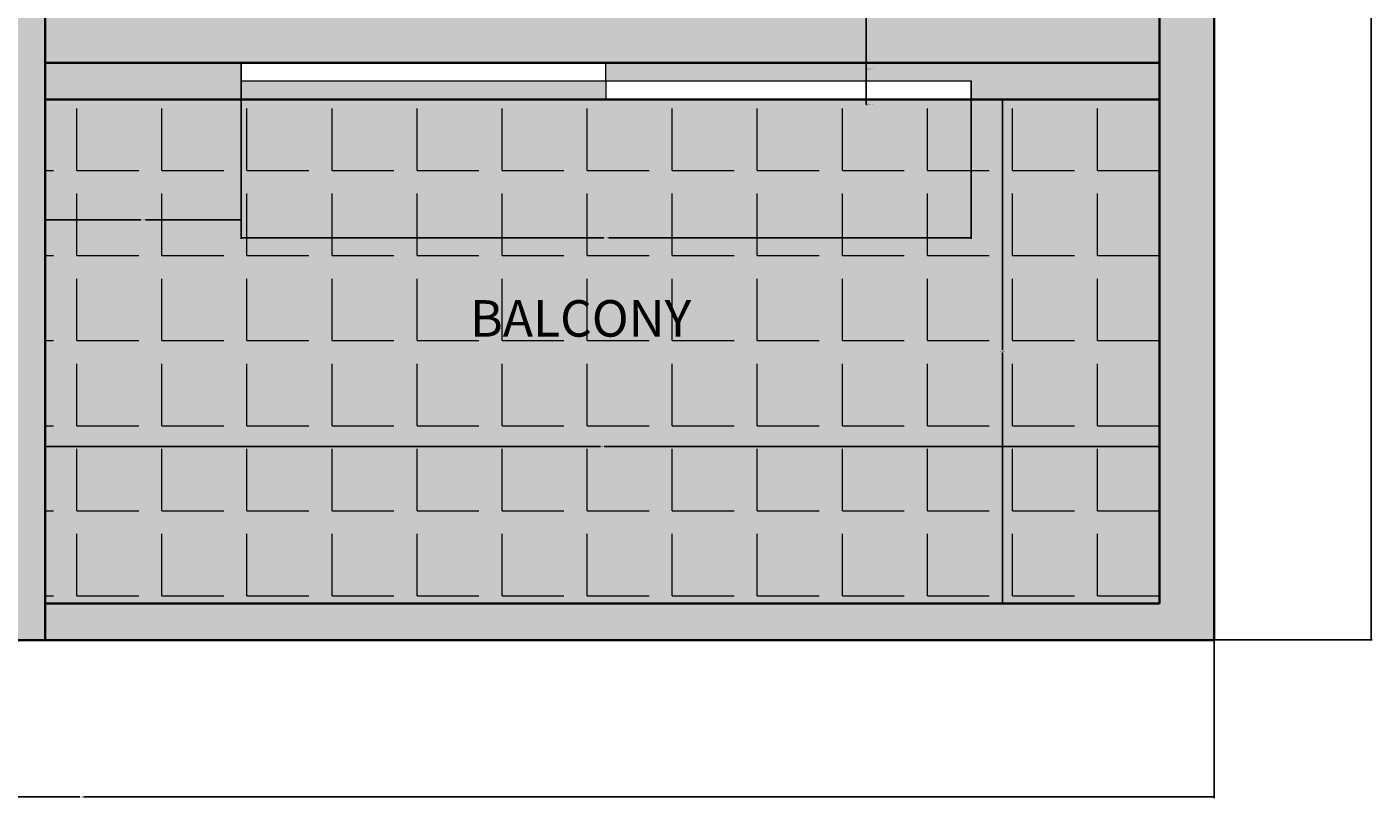
# Model space of a CAD drawing. Units: inches. Extents: x 3024 to 3952, y 1308 to 1863.
# Tile 4 of 29: x 3275 to 3496, y 1322 to 1449. Entities that reach past the tile are written whole.
import ezdxf

# ---------------------------------------------------------------- set-up
doc = ezdxf.new("R2010")
doc.units = ezdxf.units.IN
for name, color, linetype, lineweight in [('A-ANNO-DIMS', 2, 'Continuous', 18), ('A-AREA-IDEN', 7, 'Continuous', 18), ('A-DOOR', 4, 'Continuous', 18), ('A-FLOR-TILE-PATT', 7, 'Continuous', 13), ('A-WALL', 7, 'Continuous', 35)]:
    doc.layers.add(name, color=color, linetype=linetype, lineweight=lineweight)
doc.layers.add('A-FLOR-PATT', color=254, linetype='Continuous', lineweight=13, true_color=0xfeeab9)
doc.layers.add('A-WALL-PATT', color=254, linetype='Continuous', lineweight=13, true_color=0xcecce6)
doc.styles.get("Standard").update_dxf_attribs({"font": 'arial.ttf'})
doc.dimstyles.get("Standard").update_dxf_attribs({"dimtxt": 0.18, "dimasz": 0.18, "dimexe": 0.18, "dimexo": 0.0625, "dimgap": 0.09, "dimtad": 0, "dimtih": 1, "dimtoh": 1, "dimdec": 4, "dimzin": 0, "dimdsep": 46, "dimtxsty": 'Standard', "dimcen": 0.09, "dimadec": 0, "dimazin": 0, "dimtfac": 1, "dimtdec": 4, "dimtofl": 0, "dimtmove": 0, "dimatfit": 3, "dimfxl": 1, "dimtolj": 1, "dimtzin": 0, "dimarcsym": 0})

# ---------------------------------------------------------------- blocks, each defined once
blk = doc.blocks.new('*D36')
at = {"layer": 'A-ANNO-DIMS', "color": 0, "lineweight": -2, "transparency": 16777216}
for p, q in [((3097.76, 1347.78), (3097.76, 1321.89)), ((3469.76, 1347.78), (3469.76, 1321.89)), ((3097.94, 1322.07), (3283.48, 1322.07)), ((3469.58, 1322.07), (3284.05, 1322.07))]:
    blk.add_line(p, q, dxfattribs=at)
at = {"layer": 'A-ANNO-DIMS', "color": 0, "transparency": 16777216}
for points in [[(3097.94, 1322.1), (3097.94, 1322.04), (3097.76, 1322.07)], [(3469.58, 1322.1), (3469.58, 1322.04), (3469.76, 1322.07)]]:
    blk.add_solid(points, dxfattribs=at)
at = {"layer": 'Defpoints', "color": 0, "transparency": 16777216}
for p in [(3097.76, 1347.85), (3469.76, 1347.85), (3469.76, 1322.07)]:
    blk.add_point(p, dxfattribs=at)
at = {"layer": 'A-ANNO-DIMS', "color": 0, "transparency": 16777216, "insert": (3283.76, 1322.07), "char_height": 0.18, "attachment_point": 5}
blk.add_mtext('\\A1;372', dxfattribs=at)
blk = doc.blocks.new('*D37')
at = {"layer": 'A-ANNO-DIMS', "color": 0, "lineweight": -2, "transparency": 16777216}
for p, q in [((3469.83, 1787.61), (3495.72, 1787.61)), ((3495.54, 1787.43), (3495.54, 1567.91)), ((3495.54, 1348.03), (3495.54, 1567.54)), ((3469.83, 1347.85), (3495.72, 1347.85))]:
    blk.add_line(p, q, dxfattribs=at)
at = {"layer": 'A-ANNO-DIMS', "color": 0, "transparency": 16777216}
for points in [[(3495.51, 1787.43), (3495.57, 1787.43), (3495.54, 1787.61)], [(3495.51, 1348.03), (3495.57, 1348.03), (3495.54, 1347.85)]]:
    blk.add_solid(points, dxfattribs=at)
at = {"layer": 'Defpoints', "color": 0, "transparency": 16777216}
for p in [(3469.76, 1787.61), (3495.54, 1787.61), (3469.76, 1347.85)]:
    blk.add_point(p, dxfattribs=at)
at = {"layer": 'A-ANNO-DIMS', "color": 0, "transparency": 16777216, "insert": (3495.54, 1567.73), "char_height": 0.18, "attachment_point": 5}
blk.add_mtext('\\A1;439.8', dxfattribs=at)
blk = doc.blocks.new('*D46')
at = {"layer": 'A-ANNO-DIMS', "color": 0, "lineweight": -2, "transparency": 16777216}
for p, q in [((3277.76, 1353.91), (3277.76, 1379.8)), ((3277.94, 1379.62), (3368.98, 1379.62)), ((3460.58, 1379.62), (3369.54, 1379.62)), ((3460.76, 1353.91), (3460.76, 1379.8))]:
    blk.add_line(p, q, dxfattribs=at)
at = {"layer": 'A-ANNO-DIMS', "color": 0, "transparency": 16777216}
for points in [[(3277.94, 1379.65), (3277.94, 1379.59), (3277.76, 1379.62)], [(3460.58, 1379.65), (3460.58, 1379.59), (3460.76, 1379.62)]]:
    blk.add_solid(points, dxfattribs=at)
at = {"layer": 'Defpoints', "color": 0, "transparency": 16777216}
for p in [(3460.76, 1379.62), (3277.76, 1353.85), (3460.76, 1353.85)]:
    blk.add_point(p, dxfattribs=at)
at = {"layer": 'A-ANNO-DIMS', "color": 0, "transparency": 16777216, "insert": (3369.26, 1379.62), "char_height": 0.18, "attachment_point": 5}
blk.add_mtext('\\A1;183', dxfattribs=at)
blk = doc.blocks.new('*D48')
at = {"layer": 'A-ANNO-DIMS', "color": 0, "lineweight": -2, "transparency": 16777216}
for p, q in [((3460.7, 1436.61), (3434.81, 1436.61)), ((3434.99, 1436.43), (3434.99, 1395.41)), ((3434.99, 1354.03), (3434.99, 1395.04)), ((3460.7, 1353.85), (3434.81, 1353.85))]:
    blk.add_line(p, q, dxfattribs=at)
at = {"layer": 'A-ANNO-DIMS', "color": 0, "transparency": 16777216}
for points in [[(3434.96, 1436.43), (3435.02, 1436.43), (3434.99, 1436.61)], [(3434.96, 1354.03), (3435.02, 1354.03), (3434.99, 1353.85)]]:
    blk.add_solid(points, dxfattribs=at)
at = {"layer": 'Defpoints', "color": 0, "transparency": 16777216}
for p in [(3434.99, 1436.61), (3460.76, 1436.61), (3460.76, 1353.85)]:
    blk.add_point(p, dxfattribs=at)
at = {"layer": 'A-ANNO-DIMS', "color": 0, "transparency": 16777216, "insert": (3434.99, 1395.23), "char_height": 0.18, "attachment_point": 5}
blk.add_mtext('\\A1;82.76', dxfattribs=at)
blk = doc.blocks.new('*D67')
at = {"layer": 'A-ANNO-DIMS', "color": 0, "lineweight": -2, "transparency": 16777216}
for p, q in [((3309.95, 1439.61), (3309.95, 1413.71)), ((3429.86, 1439.61), (3429.86, 1413.71)), ((3310.13, 1413.89), (3369.52, 1413.89)), ((3429.68, 1413.89), (3370.29, 1413.89))]:
    blk.add_line(p, q, dxfattribs=at)
at = {"layer": 'A-ANNO-DIMS', "color": 0, "transparency": 16777216}
for points in [[(3310.13, 1413.92), (3310.13, 1413.86), (3309.95, 1413.89)], [(3429.68, 1413.92), (3429.68, 1413.86), (3429.86, 1413.89)]]:
    blk.add_solid(points, dxfattribs=at)
at = {"layer": 'Defpoints', "color": 0, "transparency": 16777216}
for p in [(3309.95, 1439.67), (3429.86, 1439.67), (3309.95, 1413.89)]:
    blk.add_point(p, dxfattribs=at)
at = {"layer": 'A-ANNO-DIMS', "color": 0, "transparency": 16777216, "insert": (3369.91, 1413.89), "char_height": 0.18, "attachment_point": 5}
blk.add_mtext('\\A1;119.9', dxfattribs=at)
blk = doc.blocks.new('*D68')
at = {"layer": 'A-ANNO-DIMS', "color": 0, "lineweight": -2, "transparency": 16777216}
for p, q in [((3277.76, 1442.54), (3277.76, 1416.65)), ((3309.95, 1442.54), (3309.95, 1416.65)), ((3277.94, 1416.83), (3293.47, 1416.83)), ((3309.77, 1416.83), (3294.25, 1416.83))]:
    blk.add_line(p, q, dxfattribs=at)
at = {"layer": 'A-ANNO-DIMS', "color": 0, "transparency": 16777216}
for points in [[(3277.94, 1416.86), (3277.94, 1416.8), (3277.76, 1416.83)], [(3309.77, 1416.86), (3309.77, 1416.8), (3309.95, 1416.83)]]:
    blk.add_solid(points, dxfattribs=at)
at = {"layer": 'Defpoints', "color": 0, "transparency": 16777216}
for p in [(3277.76, 1442.61), (3309.95, 1442.61), (3277.76, 1416.83)]:
    blk.add_point(p, dxfattribs=at)
at = {"layer": 'A-ANNO-DIMS', "color": 0, "transparency": 16777216, "insert": (3293.86, 1416.83), "char_height": 0.18, "attachment_point": 5}
blk.add_mtext('\\A1;32.19', dxfattribs=at)
blk = doc.blocks.new('*D107')
at = {"layer": 'A-ANNO-DIMS', "color": 0, "lineweight": -2, "transparency": 16777216}
for p, q in [((3412.47, 1499.22), (3412.65, 1499.22)), ((3412.56, 1499.13), (3412.56, 1499.31)), ((3412.57, 1435.78), (3412.57, 1459.39)), ((3412.75, 1435.78), (3412.57, 1435.78))]:
    blk.add_line(p, q, dxfattribs=at)
at = {"layer": 'A-ANNO-DIMS', "color": 0, "transparency": 16777216}
blk.add_solid([(3412.6, 1459.39), (3412.54, 1459.39), (3412.57, 1459.57)], dxfattribs=at)
at = {"layer": 'Defpoints', "color": 0, "transparency": 16777216}
for p in [(3412.56, 1499.22), (3412.57, 1459.57)]:
    blk.add_point(p, dxfattribs=at)
at = {"layer": 'A-ANNO-DIMS', "color": 0, "transparency": 16777216, "insert": (3413.23, 1435.78), "char_height": 0.18, "attachment_point": 5}
blk.add_mtext('\\A1;R39.65', dxfattribs=at)
blk = doc.blocks.new('*D108')
at = {"layer": 'A-ANNO-DIMS', "color": 0, "lineweight": -2, "transparency": 16777216}
for p, q in [((3412.47, 1499.97), (3412.65, 1499.97)), ((3412.56, 1499.88), (3412.56, 1500.06)), ((3412.57, 1441.65), (3412.57, 1463.34)), ((3412.75, 1441.65), (3412.57, 1441.65))]:
    blk.add_line(p, q, dxfattribs=at)
at = {"layer": 'A-ANNO-DIMS', "color": 0, "transparency": 16777216}
blk.add_solid([(3412.6, 1463.34), (3412.54, 1463.34), (3412.57, 1463.52)], dxfattribs=at)
at = {"layer": 'Defpoints', "color": 0, "transparency": 16777216}
for p in [(3412.56, 1499.97), (3412.57, 1463.52)]:
    blk.add_point(p, dxfattribs=at)
at = {"layer": 'A-ANNO-DIMS', "color": 0, "transparency": 16777216, "insert": (3413.23, 1441.65), "char_height": 0.18, "attachment_point": 5}
blk.add_mtext('\\A1;R36.45', dxfattribs=at)

msp = doc.modelspace()

# ---------------------------------------------------------------- hatches: boundary and pattern name
at = {"layer": 'A-FLOR-PATT', "transparency": 33554528}
h = msp.add_hatch(color=256, dxfattribs=at)
h.dxf.hatch_style = 1
h.paths.add_polyline_path([(3460.764, 1688.6064), (3412.764, 1688.6064), (3412.764, 1694.6064), (3460.764, 1694.6064), (3460.764, 1778.6064), (3406.764, 1778.6064), (3406.764, 1759.9514), (3318.2981, 1759.9514), (3318.2981, 1658.6064), (3322.5356, 1658.6064), (3322.5356, 1652.6064), (3292.764, 1652.6064), (3292.764, 1778.6064), (3106.764, 1778.6064), (3106.764, 1628.6064), (3172.764, 1628.6064), (3172.764, 1532.6064), (3166.764, 1532.6064), (3166.764, 1628.6064), (3106.764, 1628.6064), (3106.764, 1356.8452), (3202.812, 1356.8452), (3202.812, 1354.2534), (3202.812, 1353.8388), (3202.812, 1351.1212), (3202.812, 1347.8452), (3277.764, 1347.8452), (3277.764, 1353.8452), (3277.764, 1356.8452), (3277.764, 1442.6064), (3460.764, 1442.6064)])
h.paths.add_polyline_path([(3216.238, 1527.2064), (3216.238, 1491.2064), (3214.663, 1491.2064), (3214.663, 1491.2409, -0.39662236), (3180.243, 1526.6064), (3163.0285, 1526.6064), (3163.0285, 1531.1064), (3161.716, 1531.1064), (3161.716, 1561.1064), (3163.0285, 1561.1064), (3163.0285, 1531.1064), (3163.0285, 1526.6064), (3180.243, 1526.6064, 0.39662236), (3214.663, 1491.2409), (3214.663, 1527.2064)], flags=16)
h.paths.add_polyline_path([(3227.364, 1649.8972), (3191.364, 1649.8972), (3191.364, 1651.4722), (3227.364, 1651.4722)], flags=16)
h.paths.add_polyline_path([(3323.1172, 1606.7362), (3323.8545, 1606.8514), (3323.8545, 1594.8241), (3323.1172, 1594.9393)], flags=16)
h.paths.add_polyline_path([(3324.2232, 1606.909), (3330.1216, 1607.8307), (3330.1216, 1614.1093), (3339.3495, 1614.1093), (3340.2711, 1620.0078), (3352.4136, 1620.0078), (3353.3353, 1614.1093), (3359.9941, 1614.1093), (3360.9157, 1620.0078), (3373.0582, 1620.0078), (3373.9799, 1614.1093), (3383.2077, 1614.1093), (3383.2077, 1607.8307), (3389.1062, 1606.909), (3389.1062, 1594.7665), (3383.2077, 1593.8449), (3383.2077, 1587.5663), (3373.9799, 1587.5663), (3373.0583, 1581.6678), (3360.9157, 1581.6678), (3359.9941, 1587.5663), (3353.3353, 1587.5663), (3352.4136, 1581.6678), (3340.2711, 1581.6678), (3339.3495, 1587.5663), (3330.1216, 1587.5663), (3330.1216, 1593.8449), (3324.2232, 1594.7665)], flags=16)
h.paths.add_polyline_path([(3236.1584, 1693.1064), (3236.1584, 1723.1064), (3237.4709, 1723.1064), (3237.4709, 1693.1064)], flags=16)
h.paths.add_polyline_path([(3373.2158, 1600.6847), (3373.7965, 1600.7303), (3374.3268, 1600.7874), (3374.8132, 1600.8531), (3375.2621, 1600.9247), (3375.6801, 1600.9991), (3376.0736, 1601.0735), (3376.6855, 1601.19), (3377.366, 1601.3023), (3378.0667, 1601.3814), (3378.8026, 1601.4123), (3379.5865, 1601.3839), (3380.4537, 1601.2948), (3381.301, 1601.1717), (3382.0317, 1601.0433), (3382.4398, 1600.9607), (3382.6252, 1600.9201), (3382.919, 1600.8507), (3382.9044, 1600.8531), (3382.842, 1600.8678), (3382.7541, 1600.8896), (3382.6252, 1600.9201), (3382.4398, 1600.9607), (3382.1868, 1601.0119), (3381.8738, 1601.0711), (3381.5125, 1601.1346), (3381.1149, 1601.1988), (3380.6928, 1601.2601), (3380.2581, 1601.3149), (3379.8226, 1601.3597), (3379.3984, 1601.3908), (3378.9944, 1601.4054), (3378.6092, 1601.4042), (3378.2384, 1601.3886), (3377.8777, 1601.36), (3377.5227, 1601.32), (3377.1691, 1601.2698), (3376.8127, 1601.211), (3376.4491, 1601.145), (3376.0736, 1601.0735), (3375.4177, 1600.9494), (3374.5542, 1600.8119), (3373.5044, 1600.6988)], flags=0)
h.paths.add_polyline_path([(3380.0253, 1596.7351), (3380.499, 1596.6659), (3380.9706, 1596.6119), (3381.4375, 1596.5791), (3381.8971, 1596.5736), (3382.5886, 1596.6167), (3382.7848, 1596.6692), (3382.1465, 1596.5706), (3381.236, 1596.5815), (3380.3199, 1596.6865)], flags=0)
h.paths.add_polyline_path([(3369.6414, 1603.9617), (3370.1589, 1604.0021), (3370.6218, 1604.0539), (3371.0335, 1604.1173), (3371.3978, 1604.1921), (3371.7181, 1604.2785), (3371.9984, 1604.3761), (3372.2441, 1604.483), (3372.4611, 1604.5972), (3372.655, 1604.7163), (3372.8317, 1604.8384), (3372.9968, 1604.9611), (3373.3703, 1605.2455), (3373.8426, 1605.5328), (3374.4624, 1605.7539), (3375.1058, 1605.8302), (3375.7221, 1605.8261), (3376.4109, 1605.76), (3377.1534, 1605.6376), (3377.8945, 1605.473), (3378.1382, 1605.409), (3377.7394, 1605.5074), (3377.3509, 1605.5937), (3376.9704, 1605.6677), (3376.5999, 1605.7288), (3376.2417, 1605.7762), (3375.8979, 1605.8092), (3375.5707, 1605.8271), (3375.2621, 1605.8291), (3374.9745, 1605.8146), (3374.7092, 1605.7832), (3374.4647, 1605.7359), (3374.239, 1605.6742), (3374.0298, 1605.5996), (3373.835, 1605.5134), (3373.6525, 1605.4171), (3373.4801, 1605.3123), (3373.3156, 1605.2002), (3373.1562, 1605.0825), (3372.7603, 1604.781), (3372.236, 1604.4588), (3371.5738, 1604.2283), (3370.8493, 1604.0794), (3369.9262, 1603.976)], flags=0)
h.paths.add_polyline_path([(3366.7533, 1606.5832), (3367.1713, 1606.5519), (3367.5378, 1606.5374), (3367.8568, 1606.5394), (3368.1325, 1606.5573), (3368.3694, 1606.5903), (3368.5717, 1606.6377), (3368.7438, 1606.6988), (3368.89, 1606.7728), (3369.0146, 1606.8591), (3369.121, 1606.9568), (3369.2094, 1607.0646), (3369.2792, 1607.181), (3369.3295, 1607.3046), (3369.3596, 1607.4339), (3369.3688, 1607.5676), (3369.3565, 1607.7042), (3369.3218, 1607.8422), (3369.2649, 1607.9804), (3369.1893, 1608.1187), (3369.0993, 1608.2569), (3368.9992, 1608.3952), (3368.8934, 1608.5334), (3368.7861, 1608.6717), (3368.6817, 1608.8099), (3368.4212, 1609.1804), (3368.2685, 1609.7106), (3368.4883, 1610.1814), (3369.0537, 1610.4604), (3369.6717, 1610.5097), (3370.2812, 1610.3612), (3370.4805, 1610.2968), (3370.1882, 1610.3839), (3369.9284, 1610.4472), (3369.6905, 1610.4842), (3369.4662, 1610.4933), (3369.2555, 1610.4765), (3369.0608, 1610.4367), (3368.884, 1610.3767), (3368.7274, 1610.2994), (3368.5931, 1610.2077), (3368.4833, 1610.1045), (3368.4002, 1609.9927), (3368.3451, 1609.8747), (3368.3166, 1609.7517), (3368.3127, 1609.6244), (3368.331, 1609.4935), (3368.3696, 1609.3597), (3368.4261, 1609.2237), (3368.4985, 1609.0863), (3368.5845, 1608.9482), (3368.6817, 1608.8099), (3368.7861, 1608.6717), (3368.8934, 1608.5334), (3368.9992, 1608.3952), (3369.0993, 1608.2569), (3369.3398, 1607.8876), (3369.3941, 1607.2896), (3368.9774, 1606.7817), (3368.3928, 1606.5742), (3367.7162, 1606.5303), (3367.0044, 1606.5585)], flags=0)
h.paths.add_polyline_path([(3362.1859, 1610.2589), (3362.5478, 1610.2845), (3362.8348, 1610.3275), (3363.0585, 1610.3863), (3363.2303, 1610.4595), (3363.3619, 1610.5457), (3363.463, 1610.6432), (3363.5376, 1610.7502), (3363.5876, 1610.8643), (3363.6153, 1610.9834), (3363.6229, 1611.1055), (3363.6125, 1611.2283), (3363.5861, 1611.3496), (3363.5462, 1611.4673), (3363.4949, 1611.5797), (3363.4358, 1611.6871), (3363.3723, 1611.7902), (3363.3081, 1611.8897), (3363.2468, 1611.9863), (3363.192, 1612.0808), (3363.0258, 1612.4261), (3363.3371, 1612.8672), (3363.9008, 1612.9782), (3364.4822, 1612.9641), (3365.1098, 1612.9074), (3365.328, 1612.8805), (3364.9615, 1612.9208), (3364.6426, 1612.9496), (3364.3668, 1612.9669), (3364.1299, 1612.9726), (3363.9276, 1612.9669), (3363.7555, 1612.9496), (3363.6093, 1612.9208), (3363.4848, 1612.8805), (3363.3782, 1612.8289), (3363.2889, 1612.7672), (3363.2169, 1612.6969), (3363.1622, 1612.6193), (3363.1247, 1612.5361), (3363.1046, 1612.4484), (3363.1017, 1612.358), (3363.1161, 1612.266), (3363.1472, 1612.1738), (3363.192, 1612.0808), (3363.2468, 1611.9863), (3363.3081, 1611.8897), (3363.3723, 1611.7902), (3363.4358, 1611.6871), (3363.6363, 1611.323), (3363.5979, 1610.7003), (3363.0863, 1610.3651), (3362.3983, 1610.2622)], flags=0)
h.paths.add_polyline_path([(3352.356, 1581.2991), (3352.2408, 1580.5618), (3340.4439, 1580.5618), (3340.3287, 1581.2991)], flags=16)
h.paths.add_polyline_path([(3340.4439, 1621.1137), (3352.2408, 1621.1137), (3352.356, 1620.3764), (3340.3287, 1620.3764)], flags=16)
h.paths.add_polyline_path([(3278.4282, 1504.7424), (3290.3831, 1504.7424), (3290.3831, 1502.7499), (3291.0473, 1502.7499), (3291.0473, 1494.7799), (3290.3831, 1494.7799), (3290.3831, 1494.1158), (3291.0473, 1494.1158), (3291.0473, 1486.1458), (3290.3831, 1486.1458), (3290.3831, 1484.1533), (3291.0473, 1484.1533), (3291.0473, 1483.4892, -0.09090909), (3291.0473, 1468.8776), (3291.0473, 1468.2135), (3290.3831, 1468.2135), (3290.3831, 1464.8926), (3278.4282, 1464.8926), (3278.4282, 1472.8626), (3277.764, 1473.5268), (3277.764, 1478.84), (3278.4282, 1479.5042)], flags=16)
h.paths.add_polyline_path([(3278.7603, 1504.4103), (3290.051, 1504.4103), (3290.051, 1465.2247), (3278.7603, 1465.2247)], flags=0)
h.paths.add_polyline_path([(3123.904, 1600.7821), (3117.9039, 1602.7821), (3117.9039, 1599.7821), (3119.4039, 1599.7821), (3119.4039, 1596.7821), (3118.4039, 1596.7821), (3118.4039, 1598.7821), (3117.9039, 1598.7821), (3117.9039, 1596.2821), (3109.9039, 1596.2821), (3109.9039, 1617.2821), (3117.9039, 1617.2821), (3117.9039, 1610.7821), (3123.9038, 1612.7821, -0.70257121), (3137.9039, 1606.7822, -0.70256205)], flags=16)
h.paths.add_polyline_path([(3123.9039, 1602.7822), (3123.9039, 1610.7822, -0.73453329), (3136.9039, 1606.7822, -0.73452973)], flags=0)
h.paths.add_polyline_path([(3177.972, 1689.6473), (3109.2405, 1689.6473), (3109.2405, 1741.1959), (3177.972, 1741.1959)], flags=16)
h.paths.add_polyline_path([(3373.0006, 1581.2991), (3372.8854, 1580.5618), (3361.0885, 1580.5618), (3360.9733, 1581.2991)], flags=16)
h.paths.add_polyline_path([(3361.0885, 1621.1137), (3372.8854, 1621.1137), (3373.0006, 1620.3764), (3360.9733, 1620.3764)], flags=16)
h.paths.add_polyline_path([(3116.9039, 1598.2821, -0.41421356), (3116.1539, 1597.2821), (3111.9039, 1597.2821, -0.41421356), (3110.9039, 1598.0321), (3110.9039, 1615.2821, -0.41421356), (3111.6539, 1616.2821), (3115.9039, 1616.2821, -0.41421356), (3116.9039, 1615.5321)], flags=0)
h.paths.add_polyline_path([(3121.6122, 1728.1369), (3121.6122, 1696.5205), (3110.2715, 1696.5205), (3110.2715, 1714.3906), (3121.6122, 1714.3906), (3121.6122, 1716.4526), (3110.2715, 1716.4526), (3110.2715, 1734.3228), (3123.3304, 1734.3228), (3123.3304, 1729.8552), (3134.6711, 1741.1959), (3134.6711, 1728.1369)], flags=0)
h.paths.add_polyline_path([(3389.4748, 1606.8514), (3390.2122, 1606.7362), (3390.2122, 1594.9393), (3389.4748, 1594.8241)], flags=16)
h.paths.add_polyline_path([(3257.6842, 1762.8281), (3259.6842, 1768.8281), (3256.6842, 1768.8281), (3256.6842, 1767.3281), (3253.6842, 1767.3281), (3253.6842, 1768.3281), (3255.6842, 1768.3281), (3255.6842, 1768.8281), (3253.1842, 1768.8281), (3253.1842, 1776.8281), (3274.1842, 1776.8281), (3274.1842, 1768.8281), (3267.6842, 1768.8281), (3269.6842, 1762.8282, -0.70257121), (3263.6843, 1748.8282, -0.70256205)], flags=16)
h.paths.add_polyline_path([(3259.6842, 1762.8281), (3267.6843, 1762.8281, -0.73453329), (3263.6842, 1749.8282, -0.73452973)], flags=0)
h.paths.add_polyline_path([(3411.264, 1715.6064), (3411.264, 1716.9189), (3441.264, 1716.9189), (3441.264, 1715.6064)], flags=16)
h.paths.add_polyline_path([(3178.3806, 1449.1876), (3178.3806, 1397.639), (3109.6491, 1397.639), (3109.6491, 1449.1876)], flags=16)
h.paths.add_polyline_path([(3397.1501, 1541.7146), (3419.6183, 1541.7146), (3419.6183, 1496.7783), (3397.1501, 1496.7783)], flags=16)
h.paths.add_polyline_path([(3254.1842, 1770.5781), (3254.1842, 1774.8281, -0.41421356), (3254.9342, 1775.8281), (3272.1842, 1775.8281, -0.41421356), (3273.1842, 1775.0781), (3273.1842, 1770.8281, -0.41421356), (3272.4342, 1769.8281), (3255.1842, 1769.8281, -0.41421356)], flags=0)
h.paths.add_polyline_path([(3403.672, 1500.7601), (3403.6016, 1500.3997), (3403.5328, 1500.0441), (3403.4662, 1499.6867), (3403.4027, 1499.3226), (3403.3464, 1498.9532), (3403.3025, 1498.5811), (3403.2759, 1498.2091), (3403.2714, 1497.8401), (3403.3064, 1497.2813), (3403.3491, 1497.1219), (3403.2689, 1497.6395), (3403.2778, 1498.3719), (3403.3635, 1499.0984), (3403.4889, 1499.8168), (3403.6016, 1500.3997), (3403.672, 1500.7601), (3403.744, 1501.1315), (3403.817, 1501.5205), (3403.891, 1501.9336), (3403.9656, 1502.3769), (3404.0404, 1502.8572), (3404.115, 1503.3786), (3404.2264, 1504.2311), (3404.2571, 1504.5223), (3404.1552, 1503.6598), (3404.0063, 1502.6193), (3403.8604, 1501.7518), (3403.744, 1501.1315)], flags=0)
h.paths.add_polyline_path([(3406.5868, 1505.0416), (3406.6121, 1504.5236), (3406.6492, 1504.0526), (3406.6956, 1503.624), (3406.7491, 1503.2333), (3406.8072, 1502.8759), (3406.8676, 1502.5473), (3406.9281, 1502.243), (3407.0268, 1501.7597), (3407.1416, 1501.1368), (3407.2087, 1500.3904), (3407.1804, 1499.6703), (3407.1078, 1498.9956), (3407.0074, 1498.3199), (3406.8809, 1497.6059), (3406.7403, 1496.9627), (3406.7418, 1496.9824), (3406.7491, 1497.0249), (3406.8229, 1497.3409), (3406.8364, 1497.4025), (3406.878, 1497.6078), (3406.9261, 1497.8614), (3406.9777, 1498.1526), (3407.0298, 1498.4712), (3407.0797, 1498.8068), (3407.1243, 1499.149), (3407.1607, 1499.4874), (3407.1859, 1499.8115), (3407.1978, 1500.1137), (3407.1969, 1500.3962), (3407.1841, 1500.6642), (3407.1609, 1500.9225), (3407.1284, 1501.1761), (3407.0876, 1501.43), (3407.0398, 1501.6891), (3406.9862, 1501.9585), (3406.8832, 1502.4628), (3406.7712, 1503.0713), (3406.6657, 1503.8424), (3406.5924, 1504.7735)], flags=0)
h.paths.add_polyline_path([(3409.2517, 1507.8962), (3409.2752, 1507.4282), (3409.3079, 1507.0076), (3409.3501, 1506.6314), (3409.4015, 1506.2969), (3409.4624, 1506.0009), (3409.5326, 1505.7406), (3409.6119, 1505.5128), (3409.6988, 1505.3131), (3409.7915, 1505.1368), (3409.8883, 1504.9792), (3409.9875, 1504.8356), (3410.0872, 1504.7015), (3410.1859, 1504.572), (3410.4508, 1504.2132), (3410.7205, 1503.6035), (3410.8059, 1502.8824), (3410.7619, 1502.0875), (3410.6122, 1501.2299), (3410.4402, 1500.6169), (3410.2538, 1500.0031), (3410.0536, 1499.3219), (3409.9909, 1499.0812), (3410.1761, 1499.7472), (3410.3596, 1500.3513), (3410.4512, 1500.6561), (3410.5312, 1500.9412), (3410.6013, 1501.226), (3410.6614, 1501.512), (3410.7111, 1501.7964), (3410.7496, 1502.0763), (3410.7764, 1502.3489), (3410.7909, 1502.6114), (3410.7926, 1502.8608), (3410.7808, 1503.0944), (3410.7553, 1503.31), (3410.7169, 1503.5087), (3410.6667, 1503.6921), (3410.6061, 1503.8621), (3410.5361, 1504.0203), (3410.4578, 1504.1686), (3410.3726, 1504.3088), (3410.2815, 1504.4424), (3410.1859, 1504.572), (3410.0872, 1504.7015), (3409.859, 1505.0083), (3409.5943, 1505.5117), (3409.4266, 1506.1336), (3409.324, 1506.8011), (3409.2586, 1507.6407)], flags=0)
h.paths.add_polyline_path([(3411.4914, 1510.5878), (3411.4432, 1510.1586), (3411.4054, 1509.775), (3411.38, 1509.4354), (3411.3681, 1509.1376), (3411.3698, 1508.8784), (3411.3843, 1508.6542), (3411.4112, 1508.4618), (3411.4497, 1508.2974), (3411.4994, 1508.1575), (3411.5595, 1508.0388), (3411.6296, 1507.9375), (3411.7097, 1507.851), (3411.802, 1507.7792), (3411.9096, 1507.7225), (3412.0353, 1507.6817), (3412.1821, 1507.6572), (3412.3528, 1507.6496), (3412.5505, 1507.6597), (3412.778, 1507.6879), (3413.0364, 1507.7341), (3413.3194, 1507.7955), (3413.6188, 1507.8687), (3413.9264, 1507.95), (3414.234, 1508.036), (3414.5333, 1508.1232), (3414.8163, 1508.208), (3415.0747, 1508.287), (3415.3023, 1508.3569), (3415.5007, 1508.4158), (3415.6733, 1508.4617), (3416.1158, 1508.5538), (3416.512, 1508.2591), (3416.716, 1507.6581), (3416.61, 1507.0003), (3416.3052, 1506.3411), (3415.8928, 1505.618), (3415.7339, 1505.3633), (3415.9914, 1505.791), (3416.201, 1506.1583), (3416.3666, 1506.4739), (3416.4925, 1506.7462), (3416.5828, 1506.9838), (3416.6413, 1507.1949), (3416.6725, 1507.3883), (3416.6799, 1507.5705), (3416.6662, 1507.7417), (3416.6339, 1507.9), (3416.5851, 1508.0436), (3416.5223, 1508.1709), (3416.4478, 1508.28), (3416.3639, 1508.3692), (3416.273, 1508.4368), (3416.1765, 1508.4815), (3416.0718, 1508.5047), (3415.9553, 1508.5079), (3415.8237, 1508.493), (3415.6733, 1508.4617), (3415.5007, 1508.4158), (3415.3327, 1508.3659), (3414.6495, 1508.157), (3414.0606, 1507.9855), (3413.4456, 1507.8229), (3412.8838, 1507.701), (3412.5505, 1507.6597), (3412.0748, 1507.6354), (3411.595, 1507.8883), (3411.398, 1508.4429), (3411.3624, 1508.9927), (3411.3854, 1509.5711), (3411.4578, 1510.3071)], flags=0)
h.paths.add_polyline_path([(3135.0797, 1449.1876), (3135.0797, 1436.1286), (3122.0208, 1436.1286), (3122.0208, 1404.5122), (3110.6801, 1404.5122), (3110.6801, 1422.3823), (3122.0208, 1422.3823), (3122.0208, 1424.4443), (3110.6801, 1424.4443), (3110.6801, 1442.3145), (3123.739, 1442.3145), (3123.739, 1437.8469)], flags=0)
h.paths.add_polyline_path([(3416.4944, 1514.2949), (3416.4837, 1513.8511), (3416.4893, 1513.4867), (3416.5102, 1513.1926), (3416.5451, 1512.9593), (3416.5929, 1512.7775), (3416.6524, 1512.6379), (3416.7224, 1512.531), (3416.8017, 1512.4488), (3416.8886, 1512.3882), (3416.9813, 1512.3476), (3417.0781, 1512.3251), (3417.1773, 1512.3189), (3417.277, 1512.3274), (3417.3757, 1512.3488), (3417.4713, 1512.3813), (3417.5627, 1512.4229), (3417.65, 1512.471), (3417.7338, 1512.5225), (3417.8146, 1512.5747), (3417.8931, 1512.6245), (3417.9699, 1512.6691), (3418.2968, 1512.8265), (3418.6505, 1512.4645), (3418.7037, 1511.9342), (3418.6693, 1511.3839), (3418.6076, 1510.8228), (3418.5777, 1510.5927), (3418.6197, 1510.9333), (3418.6525, 1511.2311), (3418.6759, 1511.4903), (3418.6899, 1511.7144), (3418.6946, 1511.9069), (3418.6899, 1512.0713), (3418.6759, 1512.2112), (3418.6525, 1512.33), (3418.6197, 1512.4311), (3418.5778, 1512.5177), (3418.5276, 1512.5903), (3418.4705, 1512.6488), (3418.4075, 1512.6933), (3418.3399, 1512.7237), (3418.2686, 1512.7401), (3418.1951, 1512.7424), (3418.1204, 1512.7307), (3418.0455, 1512.7055), (3417.9792, 1512.6736), (3417.65, 1512.471), (3417.5627, 1512.4229), (3417.4713, 1512.3813), (3417.3757, 1512.3488), (3417.277, 1512.3274), (3416.878, 1512.2936), (3416.5757, 1512.7549), (3416.492, 1513.3145), (3416.4808, 1514.0384)], flags=0)
h.paths.add_polyline_path([(3392.8223, 1481.9454), (3396.7707, 1481.9454), (3396.7707, 1480.9201), (3428.3585, 1480.9201), (3428.3585, 1481.9454), (3432.3069, 1481.9454), (3432.3069, 1464.8354, -0.26666697), (3392.8223, 1464.8354)], flags=16)
h.paths.add_polyline_path([(3431.203, 1547.5428), (3450.8613, 1547.5428, -0.19047621), (3450.8614, 1484.031), (3431.203, 1484.031), (3431.203, 1488.5675), (3432.3809, 1488.5675), (3432.3809, 1543.0062), (3431.203, 1543.0062)], flags=16)
h.paths.add_polyline_path([(3451.9233, 1524.86, -0.04962821), (3451.9233, 1506.7138), (3446.7921, 1506.7138), (3446.7921, 1524.86)], flags=0)
h.paths.add_polyline_path([(3460.764, 1436.6064), (3277.764, 1436.6064), (3277.764, 1356.8452), (3277.764, 1353.8452), (3460.764, 1353.8452)], flags=17)
h.paths.add_polyline_path([(3121.3033, 1577.378), (3153.693, 1577.378), (3153.693, 1586.6752), (3121.3033, 1586.6752)], flags=24)
h.paths.add_polyline_path([(3164.1457, 1464.1276), (3210.4801, 1464.1276), (3210.4801, 1473.4247), (3164.1457, 1473.4247)], flags=24)
h.paths.add_polyline_path([(3343.1909, 1505.8863), (3373.7236, 1505.8863), (3373.7236, 1515.1773), (3343.1909, 1515.1773)], flags=24)
h.paths.add_polyline_path([(3337.6353, 1564.2926), (3370.0189, 1564.2926), (3370.0189, 1573.5836), (3337.6353, 1573.5836)], flags=24)
h.paths.add_polyline_path([(3419.204, 1753.8578), (3453.3997, 1753.8578), (3453.3997, 1762.9956), (3419.204, 1762.9956)], flags=24)
h.paths.add_polyline_path([(3341.2523, 1701.0246), (3381.0761, 1701.0246), (3381.0761, 1710.3156), (3341.2523, 1710.3156)], flags=24)
h.paths.add_polyline_path([(3245.8895, 1726.2997), (3278.2793, 1726.2997), (3278.2793, 1735.5968), (3245.8895, 1735.5968)], flags=24)
h.paths.add_polyline_path([(3128.8045, 1668.6736), (3175.1389, 1668.6736), (3175.1389, 1677.9707), (3128.8045, 1677.9707)], flags=24)
h.paths.add_polyline_path([(3345.9997, 1396.0062), (3389.09, 1396.0062), (3389.09, 1405.3033), (3345.9997, 1405.3033)], flags=24)
at = {"layer": 'A-FLOR-TILE-PATT', "transparency": 33554569}
h = msp.add_hatch(dxfattribs=at)
h.set_pattern_fill('ANGLE', color=256, scale=2)
h.set_pattern_definition([(0, (0, 0), (0, 13.97), [10.16, -3.81]), (90, (0, 0), (-13.97, 9e-16), [10.16, -3.81])])
h.paths.add_polyline_path([(3292.764, 1778.6064), (3232.764, 1778.6064), (3232.764, 1694.6064), (3236.1584, 1694.6064), (3236.1584, 1723.1064), (3237.4709, 1723.1064), (3237.4709, 1723.0777, -0.38700389), (3266.1209, 1694.6064), (3292.764, 1694.6064)])
h.paths.add_polyline_path([(3263.6843, 1748.8282, -0.70256205), (3257.6842, 1762.8281), (3259.6842, 1768.8281), (3256.6842, 1768.8281), (3256.6842, 1767.3281), (3253.6842, 1767.3281), (3253.6842, 1768.3281), (3255.6842, 1768.3281), (3255.6842, 1768.8281), (3253.1842, 1768.8281), (3253.1842, 1776.8281), (3274.1842, 1776.8281), (3274.1842, 1768.8281), (3267.6842, 1768.8281), (3269.6842, 1762.8282, -0.70257121)], flags=16)
h.paths.add_polyline_path([(3263.6842, 1749.8282, -0.73452973), (3259.6842, 1762.8281), (3267.6843, 1762.8281, -0.73453329)], flags=0)
h.paths.add_polyline_path([(3255.1842, 1769.8281, -0.41421356), (3254.1842, 1770.5781), (3254.1842, 1774.8281, -0.41421356), (3254.9342, 1775.8281), (3272.1842, 1775.8281, -0.41421356), (3273.1842, 1775.0781), (3273.1842, 1770.8281, -0.41421356), (3272.4342, 1769.8281)], flags=0)
h.paths.add_polyline_path([(3460.764, 1436.6064), (3277.764, 1436.6064), (3277.764, 1356.8452), (3277.764, 1353.8452), (3460.764, 1353.8452)])
h.paths.add_polyline_path([(3166.764, 1628.6064), (3106.764, 1628.6064), (3106.764, 1532.6064), (3133.066, 1532.6064, -0.38700389), (3161.716, 1561.0777), (3161.716, 1561.1064), (3163.0285, 1561.1064), (3163.0285, 1532.6064), (3166.764, 1532.6064)])
h.paths.add_polyline_path([(3123.904, 1600.7821), (3117.9039, 1602.7821), (3117.9039, 1599.7821), (3119.4039, 1599.7821), (3119.4039, 1596.7821), (3118.4039, 1596.7821), (3118.4039, 1598.7821), (3117.9039, 1598.7821), (3117.9039, 1596.2821), (3109.9039, 1596.2821), (3109.9039, 1617.2821), (3117.9039, 1617.2821), (3117.9039, 1610.7821), (3123.9038, 1612.7821, -0.70257121), (3137.9039, 1606.7822, -0.70256205)], flags=16)
h.paths.add_polyline_path([(3123.9039, 1602.7822), (3123.9039, 1610.7822, -0.73453329), (3136.9039, 1606.7822, -0.73452973)], flags=0)
h.paths.add_polyline_path([(3116.1539, 1597.2821), (3111.9039, 1597.2821, -0.41421356), (3110.9039, 1598.0321), (3110.9039, 1615.2821, -0.41421356), (3111.6539, 1616.2821), (3115.9039, 1616.2821, -0.41421356), (3116.9039, 1615.5321), (3116.9039, 1598.2821, -0.41421356)], flags=0)
h.paths.add_polyline_path([(3245.8895, 1726.2997), (3278.2793, 1726.2997), (3278.2793, 1735.5968), (3245.8895, 1735.5968)], flags=24)
h.paths.add_polyline_path([(3345.9997, 1396.0062), (3389.09, 1396.0062), (3389.09, 1405.3033), (3345.9997, 1405.3033)], flags=24)
h.paths.add_polyline_path([(3121.3033, 1577.378), (3153.693, 1577.378), (3153.693, 1586.6752), (3121.3033, 1586.6752)], flags=24)
at = {"layer": 'A-WALL-PATT'}
h = msp.add_hatch(color=256, dxfattribs=at)
h.dxf.hatch_style = 1
h.paths.add_polyline_path([(3106.764, 1778.6064), (3140.5977, 1778.6064), (3140.5977, 1781.8824), (3140.5977, 1784.6), (3140.5977, 1787.6064), (3097.764, 1787.6064), (3097.764, 1590.213), (3101.04, 1590.213), (3103.7576, 1590.213), (3106.764, 1590.213)])
h.paths.add_polyline_path([(3253.5314, 1781.8824), (3253.5314, 1784.6), (3253.5314, 1787.6064), (3194.6826, 1787.6064), (3194.6826, 1785.0146), (3194.6826, 1784.6), (3194.6826, 1781.8824), (3194.6826, 1778.6064), (3253.5314, 1778.6064)])
h.paths.add_polyline_path([(3333.856, 1782.2838), (3333.856, 1784.7474), (3333.856, 1787.6064), (3272.0523, 1787.6064), (3272.0523, 1785.0146), (3272.0523, 1784.6), (3272.0523, 1781.8824), (3272.0523, 1778.6064), (3333.856, 1778.6064)])
h.paths.add_polyline_path([(3428.8344, 1784.6), (3428.8344, 1787.6064), (3378.3947, 1787.6064), (3378.3947, 1784.7474), (3378.3947, 1782.2838), (3378.3947, 1778.6064), (3428.8344, 1778.6064), (3428.8344, 1781.8824)], flags=17)
h.paths.add_polyline_path([(3469.764, 1787.6064), (3451.9386, 1787.6064), (3451.9386, 1785.0146), (3451.9386, 1784.6), (3451.9386, 1781.8824), (3451.9386, 1778.6064), (3460.764, 1778.6064), (3460.764, 1353.8452), (3277.764, 1353.8452), (3277.764, 1347.8452), (3469.764, 1347.8452), (3469.764, 1353.8452)])
h.paths.add_polyline_path([(3106.764, 1571.6922), (3104.1722, 1571.6922), (3103.7576, 1571.6922), (3101.04, 1571.6922), (3097.764, 1571.6922), (3097.764, 1347.8452), (3148.7271, 1347.8452), (3148.7271, 1351.1212), (3148.7271, 1353.8388), (3148.7271, 1356.8452), (3106.764, 1356.8452)])
h.paths.add_polyline_path([(3277.764, 1532.6064), (3262.7605, 1532.6064), (3262.7605, 1582.9359), (3256.7605, 1582.9359), (3256.7605, 1532.6064), (3244.2116, 1532.6064), (3216.238, 1532.6064), (3216.238, 1527.2064), (3216.238, 1526.6064), (3271.764, 1526.6064), (3271.764, 1356.8452), (3202.812, 1356.8452), (3202.812, 1354.2534), (3202.812, 1353.8388), (3202.812, 1351.1212), (3202.812, 1347.8452), (3277.764, 1347.8452), (3277.764, 1353.8452), (3277.764, 1356.8452)])
h.paths.add_polyline_path([(3180.238, 1532.6064), (3163.0285, 1532.6064), (3163.0285, 1531.1064), (3163.0285, 1526.6064), (3180.243, 1526.6064, -0.00416688), (3180.238, 1527.2064)])
h.paths.add_polyline_path([(3133.0285, 1531.1064, -0.01250587), (3133.066, 1532.6064), (3106.764, 1532.6064), (3106.764, 1526.6064), (3133.0285, 1526.6064)], flags=17)
h.paths.add_polyline_path([(3172.764, 1628.6064), (3166.764, 1628.6064), (3166.764, 1532.6064), (3172.764, 1532.6064)])
h.paths.add_polyline_path([(3232.764, 1649.8972), (3227.364, 1649.8972), (3226.764, 1649.8972), (3226.764, 1634.6064), (3106.764, 1634.6064), (3106.764, 1628.6064), (3232.764, 1628.6064)])
h = msp.add_hatch(color=256, dxfattribs=at)
h.dxf.hatch_style = 1
h.paths.add_polyline_path([(3460.764, 1442.6064), (3369.831, 1442.6064), (3369.831, 1439.6678), (3429.8632, 1439.6678), (3429.8632, 1436.6064), (3460.764, 1436.6064)])
h.paths.add_polyline_path([(3309.9544, 1442.6064), (3277.764, 1442.6064), (3277.764, 1436.6064), (3369.831, 1436.6064), (3369.831, 1439.6678), (3309.9544, 1439.6678)])

# ---------------------------------------------------------------- linework, layer by layer
at = {"layer": 'A-DOOR'}
for p, q in [((3309.9544, 1442.6064), (3309.9544, 1439.6678)), ((3369.831, 1439.6678), (3369.831, 1442.6064)), ((3309.9544, 1439.6678), (3369.831, 1439.6678)), ((3369.831, 1439.6678), (3369.831, 1439.6678)), ((3369.831, 1439.6678), (3429.8632, 1439.6678)), ((3369.831, 1439.6678), (3369.831, 1436.6064)), ((3429.8632, 1439.6678), (3429.8632, 1436.6064))]:
    msp.add_line(p, q, dxfattribs=at)
at = {"layer": 'A-WALL'}
for p, q in [((3469.764, 1347.8452), (3469.764, 1787.6064)), ((3460.764, 1353.8452), (3460.764, 1778.6064)), ((3277.764, 1356.8452), (3277.764, 1532.6064)), ((3460.764, 1442.6064), (3277.764, 1442.6064)), ((3460.764, 1436.6064), (3277.764, 1436.6064)), ((3277.764, 1353.8452), (3277.764, 1356.8452)), ((3460.764, 1353.8452), (3277.764, 1353.8452)), ((3277.764, 1353.8452), (3277.764, 1347.8452)), ((3469.764, 1347.8452), (3469.764, 1353.8452)), ((3469.764, 1347.8452), (3097.764, 1347.8452))]:
    msp.add_line(p, q, dxfattribs=at)

# ---------------------------------------------------------------- texts
at = {"layer": 'A-AREA-IDEN'}
msp.add_text('BALCONY', height=5.98971, dxfattribs=at).set_placement((3347.5492, 1397.6579))

# ---------------------------------------------------------------- dimensions: what is measured, and where the dimension line sits
at = {"layer": 'A-ANNO-DIMS'}
for base, p1, p2, angle, override, picture, middle in [((3495.539, 1787.6064), (3469.764, 1347.8452), (3469.764, 1787.6064), 90, {"dimdec": 1, "dimlfac": 1, "dimrnd": 0, "dimzin": 0, "dimdsep": 46, "dimlunit": 2}, '*D37', (3495.539, 1567.7258)), ((3277.764, 1416.8314), (3309.9544, 1442.6064), (3277.764, 1442.6064), 180, {"dimdec": 2, "dimlfac": 1, "dimrnd": 0, "dimzin": 0, "dimdsep": 46, "dimlunit": 2}, '*D68', (3293.8592, 1416.8314)), ((3309.9544, 1413.8928), (3429.8632, 1439.6678), (3309.9544, 1439.6678), 180, {"dimdec": 1, "dimlfac": 1, "dimrnd": 0, "dimzin": 0, "dimdsep": 46, "dimlunit": 2}, '*D67', (3369.9088, 1413.8928)), ((3434.989, 1436.6064), (3460.764, 1353.8452), (3460.764, 1436.6064), 90, {"dimdec": 2, "dimlfac": 1, "dimrnd": 0, "dimzin": 0, "dimdsep": 46, "dimlunit": 2}, '*D48', (3434.989, 1395.2258))]:
    dim = msp.add_linear_dim(base=base, p1=p1, p2=p2, angle=angle, dimstyle='Standard', override=override, dxfattribs=at)
    dim.commit()
    dim.dimension.update_dxf_attribs({"geometry": picture, "text_midpoint": middle})
for center, mpoint, picture, middle in [((3412.5646, 1499.9664), (3412.565, 1463.5192), '*D108', (3413.2257, 1441.6508)), ((3412.5646, 1499.2199), (3412.565, 1459.5708), '*D107', (3413.2257, 1435.7813))]:
    dim = msp.add_radius_dim(center=center, mpoint=mpoint, dimstyle='Standard', override={"dimdec": 2, "dimlfac": 1, "dimrnd": 0, "dimzin": 0, "dimdsep": 46, "dimlunit": 2}, dxfattribs=at)
    dim.commit()
    dim.dimension.update_dxf_attribs({"geometry": picture, "text_midpoint": middle, "dimtype": 164})
for base, p1, p2, picture, middle in [((3460.764, 1379.6202), (3277.764, 1353.8452), (3460.764, 1353.8452), '*D46', (3369.264, 1379.6202)), ((3469.764, 1322.0702), (3097.764, 1347.8452), (3469.764, 1347.8452), '*D36', (3283.764, 1322.0702))]:
    dim = msp.add_linear_dim(base=base, p1=p1, p2=p2, dimstyle='Standard', override={"dimdec": 0, "dimlfac": 1, "dimrnd": 0, "dimzin": 0, "dimdsep": 46, "dimlunit": 2}, dxfattribs=at)
    dim.commit()
    dim.dimension.update_dxf_attribs({"geometry": picture, "text_midpoint": middle})

doc.saveas('drawing.dxf')
